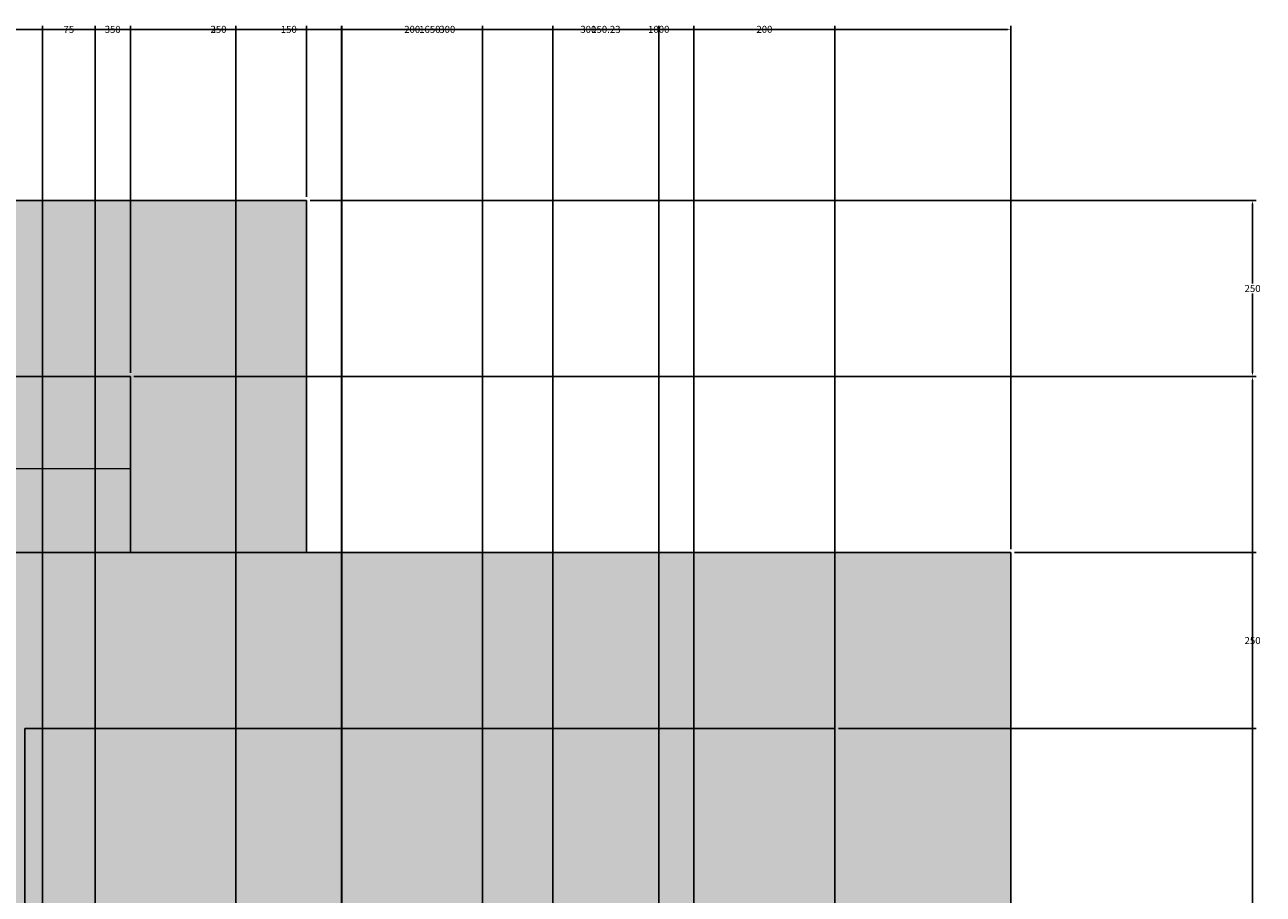
# Model space of a CAD drawing. Units: millimetres. Extents: x 2970 to 7764, y 2196 to 7505.
# Tile 13 of 13: x 6006 to 7764, y 6270 to 7505. Entities that reach past the tile are written whole.
import ezdxf

# ---------------------------------------------------------------- set-up
doc = ezdxf.new("R2010")
doc.units = ezdxf.units.MM
doc.header["$MEASUREMENT"] = 0
for name, color, linetype, lineweight in [('A-ANNO-DIMS', 2, 'Continuous', 18), ('A-ELEV', 7, 'Continuous', 25), ('A-ELEV-PATT', 8, 'Continuous', 13)]:
    doc.layers.add(name, color=color, linetype=linetype, lineweight=lineweight)
doc.styles.get("Standard").update_dxf_attribs({"font": 'arial.ttf'})
doc.dimstyles.get("Standard").update_dxf_attribs({"dimtxt": 10, "dimasz": 5, "dimexe": 5, "dimexo": 5, "dimgap": 2, "dimtad": 0, "dimtih": 1, "dimtoh": 1, "dimdec": 0, "dimzin": 0, "dimdsep": 46, "dimtxsty": 'Standard', "dimcen": 2, "dimadec": 0, "dimazin": 0, "dimtfac": 1, "dimtdec": 0, "dimtofl": 0, "dimtmove": 0, "dimatfit": 3, "dimfxl": 1, "dimtolj": 1, "dimtzin": 0, "dimarcsym": 0})

# ---------------------------------------------------------------- blocks, each defined once
blk = doc.blocks.new('*D17')
at = {"layer": 'A-ANNO-DIMS', "color": 0, "lineweight": -2, "transparency": 16777216}
for p, q in [((4555.5, 7010.8), (4555.5, 7503.8)), ((4560.5, 7498.8), (5339.1, 7498.8)), ((6150.5, 7498.8), (5371.9, 7498.8)), ((6155.5, 7010.8), (6155.5, 7503.8))]:
    blk.add_line(p, q, dxfattribs=at)
at = {"layer": 'A-ANNO-DIMS', "color": 0, "transparency": 16777216}
for points in [[(4560.5, 7499.6), (4560.5, 7498), (4555.5, 7498.8)], [(6150.5, 7499.6), (6150.5, 7498), (6155.5, 7498.8)]]:
    blk.add_solid(points, dxfattribs=at)
at = {"layer": 'Defpoints', "color": 0, "transparency": 16777216}
for p in [(6155.5, 7498.8), (4555.5, 7005.8), (6155.5, 7005.8)]:
    blk.add_point(p, dxfattribs=at)
at = {"layer": 'A-ANNO-DIMS', "color": 0, "transparency": 16777216, "insert": (5355.5, 7498.8), "char_height": 10, "attachment_point": 5}
blk.add_mtext('\\A1;1600', dxfattribs=at)
blk = doc.blocks.new('*D18')
at = {"layer": 'A-ANNO-DIMS', "color": 0, "lineweight": -2, "transparency": 16777216}
for p, q in [((6155.5, 7010.8), (6155.5, 7503.8)), ((6160.5, 7498.8), (6267.4, 7498.8)), ((6400.5, 7498.8), (6293.6, 7498.8)), ((6405.5, 7260.8), (6405.5, 7503.8))]:
    blk.add_line(p, q, dxfattribs=at)
at = {"layer": 'A-ANNO-DIMS', "color": 0, "transparency": 16777216}
for points in [[(6160.5, 7499.6), (6160.5, 7498), (6155.5, 7498.8)], [(6400.5, 7499.6), (6400.5, 7498), (6405.5, 7498.8)]]:
    blk.add_solid(points, dxfattribs=at)
at = {"layer": 'Defpoints', "color": 0, "transparency": 16777216}
for p in [(6405.5, 7498.8), (6405.5, 7255.8), (6155.5, 7005.8)]:
    blk.add_point(p, dxfattribs=at)
at = {"layer": 'A-ANNO-DIMS', "color": 0, "transparency": 16777216, "insert": (6280.5, 7498.8), "char_height": 10, "attachment_point": 5}
blk.add_mtext('\\A1;250', dxfattribs=at)
blk = doc.blocks.new('*D19')
at = {"layer": 'A-ANNO-DIMS', "color": 0, "lineweight": -2, "transparency": 16777216}
for p, q in [((6405.5, 7260.8), (6405.5, 7503.8)), ((6410.5, 7498.8), (6889.1, 7498.8)), ((7400.5, 7498.8), (6921.9, 7498.8)), ((7405.5, 6760.8), (7405.5, 7503.8))]:
    blk.add_line(p, q, dxfattribs=at)
at = {"layer": 'A-ANNO-DIMS', "color": 0, "transparency": 16777216}
for points in [[(6410.5, 7499.6), (6410.5, 7498), (6405.5, 7498.8)], [(7400.5, 7499.6), (7400.5, 7498), (7405.5, 7498.8)]]:
    blk.add_solid(points, dxfattribs=at)
at = {"layer": 'Defpoints', "color": 0, "transparency": 16777216}
for p in [(7405.5, 7498.8), (6405.5, 7255.8), (7405.5, 6755.8)]:
    blk.add_point(p, dxfattribs=at)
at = {"layer": 'A-ANNO-DIMS', "color": 0, "transparency": 16777216, "insert": (6905.5, 7498.8), "char_height": 10, "attachment_point": 5}
blk.add_mtext('\\A1;1000', dxfattribs=at)
blk = doc.blocks.new('*D32')
at = {"layer": 'A-ANNO-DIMS', "color": 0, "lineweight": -2, "transparency": 16777216}
for p, q in [((6160.5, 7005.8), (7753.5, 7005.8)), ((7748.5, 7000.8), (7748.5, 6012.9)), ((7748.5, 5010.8), (7748.5, 5998.7)), ((7410.5, 5005.8), (7753.5, 5005.8))]:
    blk.add_line(p, q, dxfattribs=at)
at = {"layer": 'A-ANNO-DIMS', "color": 0, "transparency": 16777216}
for points in [[(7747.7, 7000.8), (7749.3, 7000.8), (7748.5, 7005.8)], [(7747.7, 5010.8), (7749.3, 5010.8), (7748.5, 5005.8)]]:
    blk.add_solid(points, dxfattribs=at)
at = {"layer": 'Defpoints', "color": 0, "transparency": 16777216}
for p in [(6155.5, 7005.8), (7748.5, 7005.8), (7405.5, 5005.8)]:
    blk.add_point(p, dxfattribs=at)
at = {"layer": 'A-ANNO-DIMS', "color": 0, "transparency": 16777216, "insert": (7748.5, 6005.8), "char_height": 10, "attachment_point": 5}
blk.add_mtext('\\A1;2000', dxfattribs=at)
blk = doc.blocks.new('*D33')
at = {"layer": 'A-ANNO-DIMS', "color": 0, "lineweight": -2, "transparency": 16777216}
for p, q in [((6410.5, 7255.8), (7753.5, 7255.8)), ((7748.5, 7250.8), (7748.5, 7137.9)), ((7748.5, 7010.8), (7748.5, 7123.7)), ((6160.5, 7005.8), (7753.5, 7005.8))]:
    blk.add_line(p, q, dxfattribs=at)
at = {"layer": 'A-ANNO-DIMS', "color": 0, "transparency": 16777216}
for points in [[(7747.7, 7250.8), (7749.3, 7250.8), (7748.5, 7255.8)], [(7747.7, 7010.8), (7749.3, 7010.8), (7748.5, 7005.8)]]:
    blk.add_solid(points, dxfattribs=at)
at = {"layer": 'Defpoints', "color": 0, "transparency": 16777216}
for p in [(6405.5, 7255.8), (7748.5, 7255.8), (6155.5, 7005.8)]:
    blk.add_point(p, dxfattribs=at)
at = {"layer": 'A-ANNO-DIMS', "color": 0, "transparency": 16777216, "insert": (7748.5, 7130.8), "char_height": 10, "attachment_point": 5}
blk.add_mtext('\\A1;250', dxfattribs=at)
blk = doc.blocks.new('*D38')
at = {"layer": 'A-ANNO-DIMS', "color": 0, "lineweight": -2, "transparency": 16777216}
for p, q in [((6755.3, 4010.8), (6755.3, 7503.8)), ((6760.3, 7498.8), (6808.1, 7498.8)), ((6900.5, 7498.8), (6852.7, 7498.8)), ((6905.5, 4210.8), (6905.5, 7503.8))]:
    blk.add_line(p, q, dxfattribs=at)
at = {"layer": 'A-ANNO-DIMS', "color": 0, "transparency": 16777216}
for points in [[(6760.3, 7499.6), (6760.3, 7498), (6755.3, 7498.8)], [(6900.5, 7499.6), (6900.5, 7498), (6905.5, 7498.8)]]:
    blk.add_solid(points, dxfattribs=at)
at = {"layer": 'Defpoints', "color": 0, "transparency": 16777216}
for p in [(6905.5, 7498.8), (6905.5, 4205.8), (6755.3, 4005.8)]:
    blk.add_point(p, dxfattribs=at)
at = {"layer": 'A-ANNO-DIMS', "color": 0, "transparency": 16777216, "insert": (6830.4, 7498.8), "char_height": 10, "attachment_point": 5}
blk.add_mtext('\\A1;150.23', dxfattribs=at)
blk = doc.blocks.new('*D39')
at = {"layer": 'A-ANNO-DIMS', "color": 0, "lineweight": -2, "transparency": 16777216}
for p, q in [((5955.3, 4010.8), (5955.3, 7503.8)), ((5960.3, 7498.8), (6117.2, 7498.8)), ((6300.3, 7498.8), (6143.3, 7498.8)), ((6305.3, 4010.8), (6305.3, 7503.8))]:
    blk.add_line(p, q, dxfattribs=at)
at = {"layer": 'A-ANNO-DIMS', "color": 0, "transparency": 16777216}
for points in [[(5960.3, 7499.6), (5960.3, 7498), (5955.3, 7498.8)], [(6300.3, 7499.6), (6300.3, 7498), (6305.3, 7498.8)]]:
    blk.add_solid(points, dxfattribs=at)
at = {"layer": 'Defpoints', "color": 0, "transparency": 16777216}
for p in [(6305.3, 7498.8), (5955.3, 4005.8), (6305.3, 4005.8)]:
    blk.add_point(p, dxfattribs=at)
at = {"layer": 'A-ANNO-DIMS', "color": 0, "transparency": 16777216, "insert": (6130.3, 7498.8), "char_height": 10, "attachment_point": 5}
blk.add_mtext('\\A1;350', dxfattribs=at)
blk = doc.blocks.new('*D40')
at = {"layer": 'A-ANNO-DIMS', "color": 0, "lineweight": -2, "transparency": 16777216}
for p, q in [((6305.3, 4010.8), (6305.3, 7503.8)), ((6310.3, 7498.8), (6367.7, 7498.8)), ((6450.3, 7498.8), (6392.8, 7498.8)), ((6455.3, 4010.8), (6455.3, 7503.8))]:
    blk.add_line(p, q, dxfattribs=at)
at = {"layer": 'A-ANNO-DIMS', "color": 0, "transparency": 16777216}
for points in [[(6310.3, 7499.6), (6310.3, 7498), (6305.3, 7498.8)], [(6450.3, 7499.6), (6450.3, 7498), (6455.3, 7498.8)]]:
    blk.add_solid(points, dxfattribs=at)
at = {"layer": 'Defpoints', "color": 0, "transparency": 16777216}
for p in [(6455.3, 7498.8), (6305.3, 4005.8), (6455.3, 4005.8)]:
    blk.add_point(p, dxfattribs=at)
at = {"layer": 'A-ANNO-DIMS', "color": 0, "transparency": 16777216, "insert": (6380.3, 7498.8), "char_height": 10, "attachment_point": 5}
blk.add_mtext('\\A1;150', dxfattribs=at)
blk = doc.blocks.new('*D41')
at = {"layer": 'A-ANNO-DIMS', "color": 0, "lineweight": -2, "transparency": 16777216}
for p, q in [((6455.3, 4010.8), (6455.3, 7503.8)), ((6460.3, 7498.8), (6592.2, 7498.8)), ((6750.3, 7498.8), (6618.3, 7498.8)), ((6755.3, 4010.8), (6755.3, 7503.8))]:
    blk.add_line(p, q, dxfattribs=at)
at = {"layer": 'A-ANNO-DIMS', "color": 0, "transparency": 16777216}
for points in [[(6460.3, 7499.6), (6460.3, 7498), (6455.3, 7498.8)], [(6750.3, 7499.6), (6750.3, 7498), (6755.3, 7498.8)]]:
    blk.add_solid(points, dxfattribs=at)
at = {"layer": 'Defpoints', "color": 0, "transparency": 16777216}
for p in [(6755.3, 7498.8), (6455.3, 4005.8), (6755.3, 4005.8)]:
    blk.add_point(p, dxfattribs=at)
at = {"layer": 'A-ANNO-DIMS', "color": 0, "transparency": 16777216, "insert": (6605.3, 7498.8), "char_height": 10, "attachment_point": 5}
blk.add_mtext('\\A1;300', dxfattribs=at)
blk = doc.blocks.new('*D67')
at = {"layer": 'A-ANNO-DIMS', "color": 0, "lineweight": -2, "transparency": 16777216}
for p, q in [((5755.5, 6760.8), (5755.5, 7503.8)), ((5760.5, 7498.8), (6564.1, 7498.8)), ((7400.5, 7498.8), (6596.9, 7498.8)), ((7405.5, 6760.8), (7405.5, 7503.8))]:
    blk.add_line(p, q, dxfattribs=at)
at = {"layer": 'A-ANNO-DIMS', "color": 0, "transparency": 16777216}
for points in [[(5760.5, 7499.6), (5760.5, 7498), (5755.5, 7498.8)], [(7400.5, 7499.6), (7400.5, 7498), (7405.5, 7498.8)]]:
    blk.add_solid(points, dxfattribs=at)
at = {"layer": 'Defpoints', "color": 0, "transparency": 16777216}
for p in [(7405.5, 7498.8), (5755.5, 6755.8), (7405.5, 6755.8)]:
    blk.add_point(p, dxfattribs=at)
at = {"layer": 'A-ANNO-DIMS', "color": 0, "transparency": 16777216, "insert": (6580.5, 7498.8), "char_height": 10, "attachment_point": 5}
blk.add_mtext('\\A1;1650', dxfattribs=at)
blk = doc.blocks.new('*D69')
at = {"layer": 'A-ANNO-DIMS', "color": 0, "lineweight": -2, "transparency": 16777216}
for p, q in [((7160.5, 6505.8), (7753.5, 6505.8)), ((7748.5, 6500.8), (7748.5, 5887.9)), ((7748.5, 5260.8), (7748.5, 5873.7)), ((7160.5, 5255.8), (7753.5, 5255.8))]:
    blk.add_line(p, q, dxfattribs=at)
at = {"layer": 'A-ANNO-DIMS', "color": 0, "transparency": 16777216}
for points in [[(7747.7, 6500.8), (7749.3, 6500.8), (7748.5, 6505.8)], [(7747.7, 5260.8), (7749.3, 5260.8), (7748.5, 5255.8)]]:
    blk.add_solid(points, dxfattribs=at)
at = {"layer": 'Defpoints', "color": 0, "transparency": 16777216}
for p in [(7155.5, 6505.8), (7748.5, 6505.8), (7155.5, 5255.8)]:
    blk.add_point(p, dxfattribs=at)
at = {"layer": 'A-ANNO-DIMS', "color": 0, "transparency": 16777216, "insert": (7748.5, 5880.8), "char_height": 10, "attachment_point": 5}
blk.add_mtext('\\A1;1250', dxfattribs=at)
blk = doc.blocks.new('*D70')
at = {"layer": 'A-ANNO-DIMS', "color": 0, "lineweight": -2, "transparency": 16777216}
for p, q in [((7410.5, 6755.8), (7753.5, 6755.8)), ((7748.5, 6750.8), (7748.5, 6637.9)), ((7748.5, 6510.8), (7748.5, 6623.7)), ((7160.5, 6505.8), (7753.5, 6505.8))]:
    blk.add_line(p, q, dxfattribs=at)
at = {"layer": 'A-ANNO-DIMS', "color": 0, "transparency": 16777216}
for points in [[(7747.7, 6750.8), (7749.3, 6750.8), (7748.5, 6755.8)], [(7747.7, 6510.8), (7749.3, 6510.8), (7748.5, 6505.8)]]:
    blk.add_solid(points, dxfattribs=at)
at = {"layer": 'Defpoints', "color": 0, "transparency": 16777216}
for p in [(7405.5, 6755.8), (7748.5, 6755.8), (7155.5, 6505.8)]:
    blk.add_point(p, dxfattribs=at)
at = {"layer": 'A-ANNO-DIMS', "color": 0, "transparency": 16777216, "insert": (7748.5, 6630.8), "char_height": 10, "attachment_point": 5}
blk.add_mtext('\\A1;250', dxfattribs=at)
blk = doc.blocks.new('*D71')
at = {"layer": 'A-ANNO-DIMS', "color": 0, "lineweight": -2, "transparency": 16777216}
for p, q in [((6030.5, 6135.8), (6030.5, 7503.8)), ((6035.5, 7498.8), (6058.8, 7498.8)), ((6100.5, 7498.8), (6077.2, 7498.8)), ((6105.5, 6060.8), (6105.5, 7503.8))]:
    blk.add_line(p, q, dxfattribs=at)
at = {"layer": 'A-ANNO-DIMS', "color": 0, "transparency": 16777216}
for points in [[(6035.5, 7499.6), (6035.5, 7498), (6030.5, 7498.8)], [(6100.5, 7499.6), (6100.5, 7498), (6105.5, 7498.8)]]:
    blk.add_solid(points, dxfattribs=at)
at = {"layer": 'Defpoints', "color": 0, "transparency": 16777216}
for p in [(6105.5, 7498.8), (6030.5, 6130.8), (6105.5, 6055.8)]:
    blk.add_point(p, dxfattribs=at)
at = {"layer": 'A-ANNO-DIMS', "color": 0, "transparency": 16777216, "insert": (6068, 7498.8), "char_height": 10, "attachment_point": 5}
blk.add_mtext('\\A1;75', dxfattribs=at)
blk = doc.blocks.new('*D72')
at = {"layer": 'A-ANNO-DIMS', "color": 0, "lineweight": -2, "transparency": 16777216}
for p, q in [((6105.5, 6060.8), (6105.5, 7503.8)), ((6110.5, 7498.8), (6267.5, 7498.8)), ((6450.5, 7498.8), (6293.5, 7498.8)), ((6455.5, 6060.8), (6455.5, 7503.8))]:
    blk.add_line(p, q, dxfattribs=at)
at = {"layer": 'A-ANNO-DIMS', "color": 0, "transparency": 16777216}
for points in [[(6110.5, 7499.6), (6110.5, 7498), (6105.5, 7498.8)], [(6450.5, 7499.6), (6450.5, 7498), (6455.5, 7498.8)]]:
    blk.add_solid(points, dxfattribs=at)
at = {"layer": 'Defpoints', "color": 0, "transparency": 16777216}
for p in [(6455.5, 7498.8), (6105.5, 6055.8), (6455.5, 6055.8)]:
    blk.add_point(p, dxfattribs=at)
at = {"layer": 'A-ANNO-DIMS', "color": 0, "transparency": 16777216, "insert": (6280.5, 7498.8), "char_height": 10, "attachment_point": 5}
blk.add_mtext('\\A1;350', dxfattribs=at)
blk = doc.blocks.new('*D73')
at = {"layer": 'A-ANNO-DIMS', "color": 0, "lineweight": -2, "transparency": 16777216}
for p, q in [((6455.5, 6060.8), (6455.5, 7503.8)), ((6460.5, 7498.8), (6542.4, 7498.8)), ((6650.5, 7498.8), (6568.6, 7498.8)), ((6655.5, 5960.8), (6655.5, 7503.8))]:
    blk.add_line(p, q, dxfattribs=at)
at = {"layer": 'A-ANNO-DIMS', "color": 0, "transparency": 16777216}
for points in [[(6460.5, 7499.6), (6460.5, 7498), (6455.5, 7498.8)], [(6650.5, 7499.6), (6650.5, 7498), (6655.5, 7498.8)]]:
    blk.add_solid(points, dxfattribs=at)
at = {"layer": 'Defpoints', "color": 0, "transparency": 16777216}
for p in [(6655.5, 7498.8), (6455.5, 6055.8), (6655.5, 5955.8)]:
    blk.add_point(p, dxfattribs=at)
at = {"layer": 'A-ANNO-DIMS', "color": 0, "transparency": 16777216, "insert": (6555.5, 7498.8), "char_height": 10, "attachment_point": 5}
blk.add_mtext('\\A1;200', dxfattribs=at)
blk = doc.blocks.new('*D74')
at = {"layer": 'A-ANNO-DIMS', "color": 0, "lineweight": -2, "transparency": 16777216}
for p, q in [((6655.5, 5960.8), (6655.5, 7503.8)), ((6660.5, 7498.8), (6792.5, 7498.8)), ((6950.5, 7498.8), (6818.5, 7498.8)), ((6955.5, 5960.8), (6955.5, 7503.8))]:
    blk.add_line(p, q, dxfattribs=at)
at = {"layer": 'A-ANNO-DIMS', "color": 0, "transparency": 16777216}
for points in [[(6660.5, 7499.6), (6660.5, 7498), (6655.5, 7498.8)], [(6950.5, 7499.6), (6950.5, 7498), (6955.5, 7498.8)]]:
    blk.add_solid(points, dxfattribs=at)
at = {"layer": 'Defpoints', "color": 0, "transparency": 16777216}
for p in [(6955.5, 7498.8), (6655.5, 5955.8), (6955.5, 5955.8)]:
    blk.add_point(p, dxfattribs=at)
at = {"layer": 'A-ANNO-DIMS', "color": 0, "transparency": 16777216, "insert": (6805.5, 7498.8), "char_height": 10, "attachment_point": 5}
blk.add_mtext('\\A1;300', dxfattribs=at)
blk = doc.blocks.new('*D75')
at = {"layer": 'A-ANNO-DIMS', "color": 0, "lineweight": -2, "transparency": 16777216}
for p, q in [((6955.5, 5960.8), (6955.5, 7503.8)), ((6960.5, 7498.8), (7042.4, 7498.8)), ((7150.5, 7498.8), (7068.6, 7498.8)), ((7155.5, 5260.8), (7155.5, 7503.8))]:
    blk.add_line(p, q, dxfattribs=at)
at = {"layer": 'A-ANNO-DIMS', "color": 0, "transparency": 16777216}
for points in [[(6960.5, 7499.6), (6960.5, 7498), (6955.5, 7498.8)], [(7150.5, 7499.6), (7150.5, 7498), (7155.5, 7498.8)]]:
    blk.add_solid(points, dxfattribs=at)
at = {"layer": 'Defpoints', "color": 0, "transparency": 16777216}
for p in [(7155.5, 7498.8), (6955.5, 5955.8), (7155.5, 5255.8)]:
    blk.add_point(p, dxfattribs=at)
at = {"layer": 'A-ANNO-DIMS', "color": 0, "transparency": 16777216, "insert": (7055.5, 7498.8), "char_height": 10, "attachment_point": 5}
blk.add_mtext('\\A1;200', dxfattribs=at)

msp = doc.modelspace()

# ---------------------------------------------------------------- hatches: boundary and pattern name
at = {"layer": 'A-ELEV-PATT'}
h = msp.add_hatch(color=256, dxfattribs=at)
h.dxf.hatch_style = 1
h.paths.add_polyline_path([(6405.5, 7255.789), (4305.5, 7255.789), (4305.5, 6505.789), (3730.5, 6505.789), (3730.5, 4205.789), (3730.5, 2945.789), (3730.5, 2895.789), (3830.5, 2895.789), (3830.5, 4205.789), (3830.5, 6405.789), (4405.5, 6405.789), (4405.5, 4205.789), (6905.5, 4205.789), (6905.5, 2945.789), (6905.5, 2845.789), (7155.5, 2845.789), (7155.5, 2945.789), (7155.5, 4205.789), (7155.5, 4455.789), (4555.5, 4455.789), (4555.5, 6505.789), (4555.5, 7005.789), (6155.5, 7005.789), (6155.5, 6755.789), (6405.5, 6755.789)])
h.paths.add_polyline_path([(7405.5, 6755.789), (6155.5, 6755.789), (5755.5, 6755.789), (5755.5, 5005.789), (7405.5, 5005.789)])
h.paths.add_polyline_path([(7155.5, 6505.789), (7155.5, 5255.789), (6005.5, 5255.789), (6005.5, 6505.789)], flags=16)
h.paths.add_polyline_path([(6105.5, 5520.789), (6105.5, 6055.789), (6455.5, 6055.789), (6455.5, 5520.789), (6655.5, 5520.789), (6655.5, 5605.789), (6655.5, 5955.789), (6955.5, 5955.789), (6955.5, 5605.789), (6955.5, 5520.789)], flags=0)
h.paths.add_polyline_path([(6425.5, 5755.789), (6425.5, 5655.789), (6425.5, 5555.789), (6405.5, 5555.789), (6405.5, 5755.789)], flags=0)
h.paths.add_polyline_path([(6955.5, 5505.789), (6955.5, 5405.789), (6655.5, 5405.789), (6655.5, 5505.789)], flags=0)
h = msp.add_hatch(color=256, dxfattribs=at)
h.set_gradient(color1=(147, 149, 152), color2=(199, 200, 202), name='CURVED')
h.paths.add_polyline_path([(6955.5, 4455.789), (6955.5, 5005.789), (5755.5, 5005.789), (5755.5, 6755.789), (6155.5, 6755.789), (6155.5, 7005.789), (4555.5, 7005.789), (4555.5, 6505.789), (4555.5, 4455.789)])
h.paths.add_polyline_path([(5015.81, 5462.49), (5015.81, 6062.49), (5455.81, 6062.49), (5455.81, 5462.49)], flags=16)
h.paths.add_polyline_path([(5035.81, 5482.49), (5035.81, 6042.49), (5155.81, 6042.49), (5155.81, 5482.49)], flags=0)
h.paths.add_polyline_path([(5175.81, 5482.49), (5175.81, 6042.49), (5295.81, 6042.49), (5295.81, 5482.49)], flags=0)
h.paths.add_polyline_path([(5315.81, 5482.49), (5315.81, 6042.49), (5435.81, 6042.49), (5435.81, 5482.49)], flags=0)
h.paths.add_polyline_path([(4865.81, 6162.49), (4865.81, 6212.49), (4840.81, 6212.49), (4840.81, 6237.49), (5630.81, 6237.49), (5630.81, 6212.49), (5605.81, 6212.49), (5605.81, 6162.49), (5015.81, 6162.49)], flags=16)
h = msp.add_hatch(dxfattribs=at)
h.set_pattern_fill('ANSI31', color=256, scale=1250, angle=135, style=0)
h.paths.add_polyline_path([(5755.5, 6755.789), (6155.5, 6755.789), (6155.5, 7005.789), (4555.5, 7005.789), (4555.5, 6505.789), (4555.5, 4455.789), (6955.5, 4455.789), (6955.5, 5005.789), (5755.5, 5005.789)])
h.paths.add_polyline_path([(5015.81, 5462.49), (5015.81, 6062.49), (5455.81, 6062.49), (5455.81, 5462.49)], flags=16)
h.paths.add_polyline_path([(5035.81, 5482.49), (5035.81, 6042.49), (5155.81, 6042.49), (5155.81, 5482.49)], flags=0)
h.paths.add_polyline_path([(5175.81, 5482.49), (5175.81, 6042.49), (5295.81, 6042.49), (5295.81, 5482.49)], flags=0)
h.paths.add_polyline_path([(5315.81, 5482.49), (5315.81, 6042.49), (5435.81, 6042.49), (5435.81, 5482.49)], flags=0)
h.paths.add_polyline_path([(4865.81, 6162.49), (4865.81, 6212.49), (4840.81, 6212.49), (4840.81, 6237.49), (5630.81, 6237.49), (5630.81, 6212.49), (5605.81, 6212.49), (5605.81, 6162.49), (5015.81, 6162.49)], flags=16)
h = msp.add_hatch(color=256, dxfattribs=at)
h.set_gradient(color1=(19, 76, 0), color2=(0, 127, 31), name='INVCURVED')
h.paths.add_polyline_path([(6005.5, 6505.789), (6005.5, 6230.789), (7155.5, 6230.789), (7155.5, 6505.789)])

# ---------------------------------------------------------------- linework, layer by layer
at = {"layer": 'A-ELEV'}
for p, q in [((4305.5, 7255.789), (6405.5, 7255.789)), ((6405.5, 7255.789), (6405.5, 6755.789)), ((4555.5, 7005.789), (6155.5, 7005.789)), ((6155.5, 7005.789), (6155.5, 6755.789)), ((5755.5, 6755.789), (6155.5, 6755.789)), ((6155.5, 6755.789), (7405.5, 6755.789)), ((7405.5, 6755.789), (7405.5, 5005.789)), ((6005.5, 6505.789), (7155.5, 6505.789)), ((6005.5, 5255.789), (6005.5, 6505.789)), ((7155.5, 6505.789), (7155.5, 5255.789))]:
    msp.add_line(p, q, dxfattribs=at)

# ---------------------------------------------------------------- dimensions: what is measured, and where the dimension line sits
at = {"layer": 'A-ANNO-DIMS'}
for base, p1, p2, override, picture, middle in [((6155.5, 7498.789), (4555.5, 7005.789), (6155.5, 7005.789), {"dimdec": 0, "dimlfac": 1, "dimrnd": 0, "dimzin": 0, "dimdsep": 46, "dimlunit": 2}, '*D17', (5355.5, 7498.789)), ((7405.5, 7498.789), (5755.5, 6755.789), (7405.5, 6755.789), {"dimdec": 0, "dimlfac": 1, "dimrnd": 0, "dimzin": 0, "dimdsep": 46, "dimlunit": 2}, '*D67', (6580.5, 7498.789)), ((6305.271, 7498.789), (5955.271, 4005.789), (6305.271, 4005.789), {"dimdec": 0, "dimlfac": 1, "dimrnd": 0, "dimzin": 0, "dimdsep": 46, "dimlunit": 2}, '*D39', (6130.271, 7498.789)), ((6105.5, 7498.789), (6030.5, 6130.789), (6105.5, 6055.789), {"dimdec": 0, "dimlfac": 1, "dimrnd": 0, "dimzin": 0, "dimdsep": 46, "dimlunit": 2}, '*D71', (6068, 7498.789)), ((6455.5, 7498.789), (6105.5, 6055.789), (6455.5, 6055.789), {"dimdec": 0, "dimlfac": 1, "dimrnd": 0, "dimzin": 0, "dimdsep": 46, "dimlunit": 2}, '*D72', (6280.5, 7498.789)), ((6405.5, 7498.789), (6155.5, 7005.789), (6405.5, 7255.789), {"dimdec": 0, "dimlfac": 1, "dimrnd": 0, "dimzin": 0, "dimdsep": 46, "dimlunit": 2}, '*D18', (6280.5, 7498.789)), ((6455.271, 7498.789), (6305.271, 4005.789), (6455.271, 4005.789), {"dimdec": 0, "dimlfac": 1, "dimrnd": 0, "dimzin": 0, "dimdsep": 46, "dimlunit": 2}, '*D40', (6380.271, 7498.789)), ((7405.5, 7498.789), (6405.5, 7255.789), (7405.5, 6755.789), {"dimdec": 0, "dimlfac": 1, "dimrnd": 0, "dimzin": 0, "dimdsep": 46, "dimlunit": 2}, '*D19', (6905.5, 7498.789)), ((6755.271, 7498.789), (6455.271, 4005.789), (6755.271, 4005.789), {"dimdec": 0, "dimlfac": 1, "dimrnd": 0, "dimzin": 0, "dimdsep": 46, "dimlunit": 2}, '*D41', (6605.271, 7498.789)), ((6655.5, 7498.789), (6455.5, 6055.789), (6655.5, 5955.789), {"dimdec": 0, "dimlfac": 1, "dimrnd": 0, "dimzin": 0, "dimdsep": 46, "dimlunit": 2}, '*D73', (6555.5, 7498.789)), ((6955.5, 7498.789), (6655.5, 5955.789), (6955.5, 5955.789), {"dimdec": 0, "dimlfac": 1, "dimrnd": 0, "dimzin": 0, "dimdsep": 46, "dimlunit": 2}, '*D74', (6805.5, 7498.789)), ((6905.5, 7498.789), (6755.271, 4005.789), (6905.5, 4205.789), {"dimdec": 2, "dimlfac": 1, "dimrnd": 0, "dimzin": 0, "dimdsep": 46, "dimlunit": 2}, '*D38', (6830.386, 7498.789)), ((7155.5, 7498.789), (6955.5, 5955.789), (7155.5, 5255.789), {"dimdec": 0, "dimlfac": 1, "dimrnd": 0, "dimzin": 0, "dimdsep": 46, "dimlunit": 2}, '*D75', (7055.5, 7498.789))]:
    dim = msp.add_linear_dim(base=base, p1=p1, p2=p2, dimstyle='Standard', override=override, dxfattribs=at)
    dim.commit()
    dim.dimension.update_dxf_attribs({"geometry": picture, "text_midpoint": middle})
for base, p1, p2, picture, middle in [((7748.5, 7255.789), (6155.5, 7005.789), (6405.5, 7255.789), '*D33', (7748.5, 7130.789)), ((7748.5, 7005.789), (7405.5, 5005.789), (6155.5, 7005.789), '*D32', (7748.5, 6005.789)), ((7748.5, 6755.789), (7155.5, 6505.789), (7405.5, 6755.789), '*D70', (7748.5, 6630.789)), ((7748.5, 6505.789), (7155.5, 5255.789), (7155.5, 6505.789), '*D69', (7748.5, 5880.789))]:
    dim = msp.add_linear_dim(base=base, p1=p1, p2=p2, angle=90, dimstyle='Standard', override={"dimdec": 0, "dimlfac": 1, "dimrnd": 0, "dimzin": 0, "dimdsep": 46, "dimlunit": 2}, dxfattribs=at)
    dim.commit()
    dim.dimension.update_dxf_attribs({"geometry": picture, "text_midpoint": middle})

doc.saveas('drawing.dxf')
